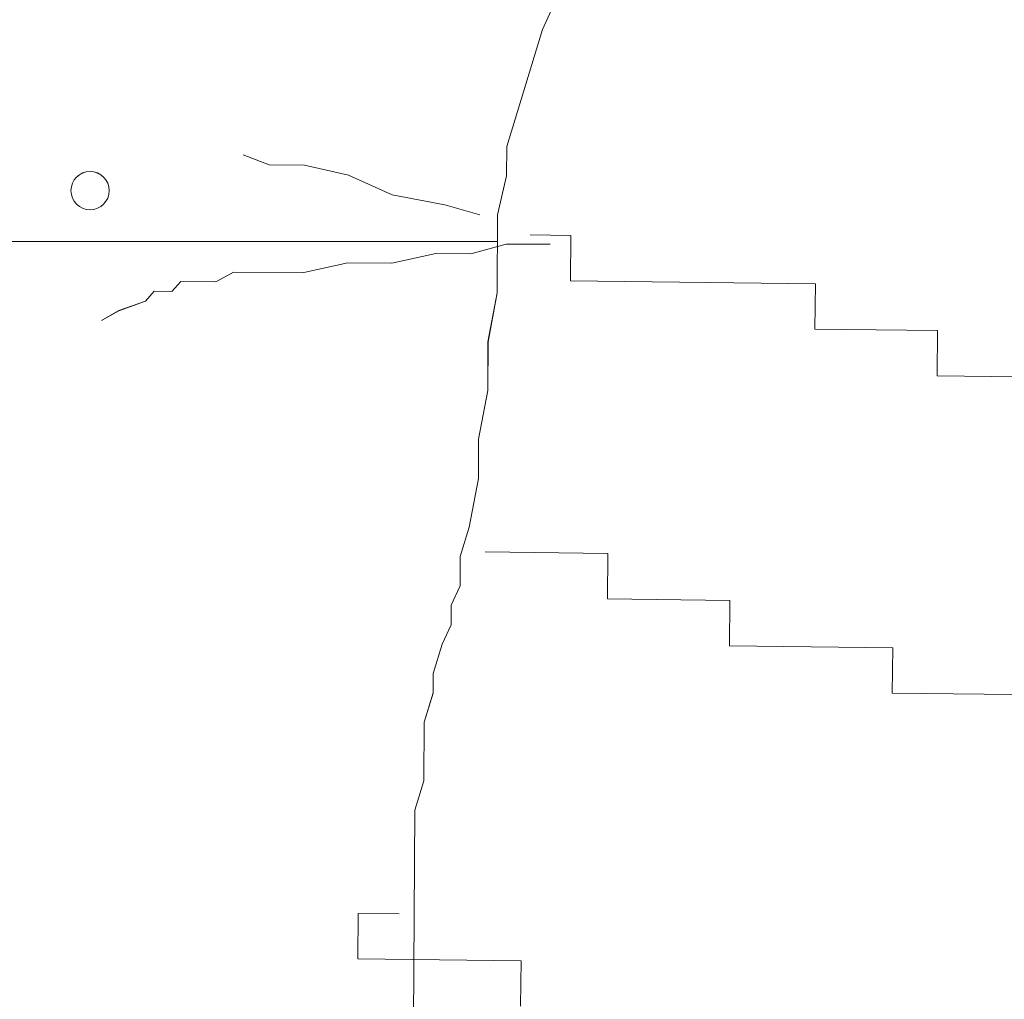
# Model space of a CAD drawing. Units: inches. Extents: x -466983 to 1020, y 324 to 318697.
# Tile 59 of 97: x 631.804 to 634.801, y 942.694 to 945.675. Entities that reach past the tile are written whole.
import ezdxf

# ---------------------------------------------------------------- set-up
doc = ezdxf.new("R2010")
doc.units = ezdxf.units.IN
doc.header["$MEASUREMENT"] = 0
doc.layers.add('A-FLOR-PATT', color=252, linetype='Continuous', lineweight=13)
doc.layers.add('A-FURN', color=8, linetype='Continuous', lineweight=18)

# ---------------------------------------------------------------- blocks, each defined once
blk = doc.blocks.new('L Shaped Sofa')
at = {"ltscale": 2}
for p, q in [((2438.4141, 742.6892), (2438.4273, 744.8578)), ((2437.8266, 743.7781), (2437.8235, 743.5262)), ((2437.8235, 743.5262), (2438.7308, 743.5151)), ((2438.7308, 743.5151), (2438.7278, 743.2632)), ((2438.7278, 743.2632), (2438.5009, 743.2659)), ((2438.3643, 742.5267), (2438.4141, 742.6892)), ((2438.3623, 742.2015), (2438.3643, 742.5267)), ((2438.3125, 742.039), (2438.3623, 742.2015)), ((2435.083, 742.048), (2435.7635, 742.0396)), ((2435.7635, 742.0396), (2435.7604, 741.7877)), ((2438.3118, 741.9306), (2438.3125, 742.039)), ((2438.262, 741.7682), (2438.3118, 741.9306)), ((2435.7604, 741.7877), (2436.6678, 741.7766)), ((2436.6678, 741.7766), (2436.6647, 741.5247)), ((2438.2126, 741.66), (2438.262, 741.7682)), ((2438.2119, 741.5515), (2438.2126, 741.66)), ((2438.1624, 741.4433), (2438.2119, 741.5515)), ((2436.6647, 741.5247), (2437.3452, 741.5164)), ((2437.3452, 741.5164), (2437.3421, 741.2645)), ((2438.1615, 741.2807), (2438.1624, 741.4433)), ((2438.1117, 741.1183), (2438.1615, 741.2807)), ((2437.3421, 741.2645), (2438.0226, 741.2562)), ((2438.0612, 740.8474), (2438.1117, 741.1183)), ((2438.0599, 740.6306), (2438.0612, 740.8474)), ((2438.0094, 740.3597), (2438.0599, 740.6306)), ((2438.0078, 740.0886), (2438.0094, 740.3597)), ((2435.0614, 740.2846), (2435.5151, 740.279)), ((2435.5151, 740.279), (2435.512, 740.0271)), ((2437.9573, 739.8178), (2438.0078, 740.0886)), ((2435.512, 740.0271), (2436.1926, 740.0188)), ((2436.1926, 740.0188), (2436.1895, 739.7669)), ((2440.0562, 739.9164), (2440.1541, 739.9701)), ((2439.9094, 739.8628), (2440.0562, 739.9164)), ((2439.8603, 739.8089), (2439.9094, 739.8628)), ((2437.9547, 739.3841), (2437.9573, 739.8178)), ((2439.7136, 739.7553), (2439.7627, 739.8093)), ((2439.7627, 739.8093), (2439.8603, 739.8089)), ((2436.1895, 739.7669), (2437.5505, 739.7503)), ((2437.5505, 739.7503), (2437.5474, 739.4984)), ((2439.4205, 739.7025), (2439.5184, 739.7562)), ((2439.5184, 739.7562), (2439.7136, 739.7553)), ((2438.7858, 739.6512), (2439.0301, 739.7043)), ((2439.0301, 739.7043), (2439.4205, 739.7025)), ((2438.2975, 739.5993), (2438.5419, 739.6524)), ((2438.5419, 739.6524), (2438.7858, 739.6512)), ((2437.9069, 739.5469), (2438.1024, 739.6002)), ((2438.1024, 739.6002), (2438.2975, 739.5993)), ((2437.6629, 739.5481), (2437.9069, 739.5469)), ((2458.9601, 739.5321), (2437.9556, 739.5321)), ((2437.5474, 739.4984), (2437.7743, 739.4956)), ((2437.9045, 739.1674), (2437.9547, 739.3841)), ((2438.0522, 739.3836), (2438.2471, 739.3285)), ((2438.2471, 739.3285), (2438.5395, 739.2729)), ((2438.5395, 739.2729), (2438.7828, 739.1633)), ((2437.9035, 739.0048), (2437.9045, 739.1674)), ((2438.7828, 739.1633), (2439.0265, 739.1079)), ((2439.0265, 739.1079), (2439.2217, 739.107)), ((2439.2217, 739.107), (2439.3677, 739.0521)), ((2437.7044, 738.3551), (2437.9035, 739.0048)), ((2437.6549, 738.2469), (2437.7044, 738.3551))]:
    blk.add_line(p, q, dxfattribs=at)
for start, end in [(90, 270), (270, 90)]:
    blk.add_arc((2440.2165, 739.2499), 0.1062, start, end, dxfattribs=at)

msp = doc.modelspace()

# ---------------------------------------------------------------- hatches: boundary and pattern name
at = {"layer": 'A-FLOR-PATT', "transparency": 33554572}
h = msp.add_hatch(dxfattribs=at)
h.set_pattern_fill('ANSI37', color=256, scale=30)
h.set_pattern_definition([(45, (-1212.4137, -290.035), (-2.6516504, 2.6516504), []), (135, (-1212.4137, -290.035), (-2.6516504, -2.6516504), [])])
h.paths.add_polyline_path([(901.8057, 1075.9377), (900.6144, 1075.9377), (900.6144, 1065.3856), (899.391, 1065.3856), (898.0911, 1065.3856), (892.8356, 1058.7098, -0.258377), (892.1875, 1058.3509), (879.9848, 1058.3509, -0.20177), (879.4382, 1058.5808), (874.0812, 1065.3856), (872.7813, 1065.3856), (871.5579, 1065.3856), (871.5579, 1075.9377), (813.8057, 1075.9377), (813.8057, 1044.7922), (832.3947, 1044.7922, -0.394795), (848.6602, 1028.5356), (848.6602, 1009.9377), (901.8057, 1009.9377), (901.8057, 1015.9377), (901.3057, 1015.9377), (871.3057, 1015.9377), (871.3057, 1017.2502), (871.3344, 1017.2502, -0.401453), (901.3057, 1045.9377), (901.8057, 1045.9377)])
edge = h.paths.add_edge_path(flags=16)
edge.add_line((847.7731, 1068.9486), (847.7731, 1073.7088))
edge.add_arc((849.2269, 1073.7088), 1.4538, 90, 180, ccw=False)
edge.add_line((849.2269, 1075.1627), (864.4921, 1075.1627))
edge.add_arc((864.4921, 1073.7088), 1.4538, 0, 90, ccw=False)
edge.add_line((865.9459, 1073.7088), (865.9459, 1069.0035))
edge.add_arc((832.6447, 1068.9761), 33.3012, -20.61234, 0.04725, ccw=False)
edge.add_ellipse((856.8595, 1058.48), major_axis=(0, 10.2131), ratio=0.6859192, start_angle=100.00884, end_angle=259.99116, ccw=False)
edge.add_arc((881.0742, 1068.9761), 33.3012, 180.04725, 200.61234, ccw=False)
h.paths.add_polyline_path([(853.1456, 1066.4815), (853.1456, 1066.4534), (853.1463, 1066.4534, 0.433107), (852.9166, 1066.6849), (852.9166, 1066.4534), (853.1456, 1066.4534), (853.1456, 1066.4815), (853.088, 1066.6122, 0.697939), (852.6995, 1066.4534), (852.7003, 1066.4534), (852.7003, 1066.4815), (852.9166, 1067.0012), (852.9166, 1066.6849, -0.396254)], flags=0)
h.paths.add_polyline_path([(861.0187, 1066.4815), (861.0187, 1066.4534), (861.0194, 1066.4534, 0.416404), (860.8024, 1066.6849), (860.8024, 1066.4534), (861.0187, 1066.4534), (861.0187, 1066.4815), (860.9672, 1066.6053, 0.713344), (860.5726, 1066.4534), (860.5734, 1066.4534), (860.5734, 1066.4815), (860.8024, 1067.0012), (860.8024, 1066.6849, -0.379973)], flags=0)
edge = h.paths.add_edge_path(flags=0)
edge.add_spline(control_points=[(861.1298, 1065.7855), (861.4661, 1065.2478), (861.6134, 1065.0161), (861.9833, 1064.3736), (862.1924, 1063.9443), (862.5614, 1063.0391), (862.7212, 1062.5633), (862.9865, 1061.5781), (863.092, 1061.0689), (863.2452, 1060.031), (863.293, 1059.5025), (863.3295, 1058.4409), (863.3181, 1057.9078), (863.2366, 1056.8518), (863.1664, 1056.3289), (862.9695, 1055.308), (862.8427, 1054.8099), (862.5365, 1053.8522), (862.3571, 1053.3927), (861.9514, 1052.5249), (861.7251, 1052.1166), (861.233, 1051.3622), (860.9672, 1051.0162), (860.4048, 1050.3949), (860.1082, 1050.1197), (859.4937, 1049.6461), (859.1758, 1049.4476), (858.5276, 1049.1299), (858.1973, 1049.0107), (857.5315, 1048.8518), (857.1959, 1048.8121), (856.5249, 1048.812), (856.1894, 1048.8515), (855.5236, 1049.0101), (855.1933, 1049.1291), (854.545, 1049.4465), (854.2271, 1049.6449), (853.6124, 1050.1183), (853.3158, 1050.3933), (852.7533, 1051.0143), (852.4874, 1051.3602), (851.9952, 1052.1144), (851.7688, 1052.5225), (851.3629, 1053.3902), (851.1834, 1053.8496), (850.877, 1054.8071), (850.7501, 1055.3051), (850.553, 1056.326), (850.4827, 1056.8488), (850.401, 1057.9048), (850.3895, 1058.4379), (850.4257, 1059.4995), (850.4734, 1060.0281), (850.6265, 1061.066), (850.7318, 1061.5753), (850.9969, 1062.5605), (851.1567, 1063.0365), (851.5254, 1063.9418), (851.7345, 1064.3712), (852.1056, 1065.0164), (852.2544, 1065.2503), (852.6082, 1065.7335)], knot_values=[3.915332, 3.915332, 3.915332, 3.915332, 4.013468, 4.013468, 4.175532, 4.175532, 4.337596, 4.337596, 4.49966, 4.49966, 4.661724, 4.661724, 4.823788, 4.823788, 4.985852, 4.985852, 5.147916, 5.147916, 5.30998, 5.30998, 5.472044, 5.472044, 5.634109, 5.634109, 5.796173, 5.796173, 5.958237, 5.958237, 6.120301, 6.120301, 6.282365, 6.282365, 6.444429, 6.444429, 6.606493, 6.606493, 6.768557, 6.768557, 6.930621, 6.930621, 7.092685, 7.092685, 7.254749, 7.254749, 7.416813, 7.416813, 7.578878, 7.578878, 7.740942, 7.740942, 7.903006, 7.903006, 8.06507, 8.06507, 8.227134, 8.227134, 8.389198, 8.389198, 8.551262, 8.551262, 8.65037, 8.65037, 8.65037, 8.65037], degree=3, periodic=0)
edge.add_line((852.6421, 1065.7855), (861.1298, 1065.7855))
edge = h.paths.add_edge_path(flags=0)
edge.add_ellipse((856.8496, 1057.7432), major_axis=(0, 7.7921), ratio=0.687861, start_angle=0, end_angle=360)
h.paths.add_polyline_path([(848.8634, 1069.3891), (848.8634, 1073.9605, -0.414214), (849.9538, 1075.0508), (863.7652, 1075.0508, -0.414214), (864.8555, 1073.9605), (864.8555, 1069.3891, -0.388936), (864.5237, 1069.027, -0.043561), (849.1953, 1069.027, -0.388936)], flags=0)
h.paths.add_polyline_path([(853.1006, 1068.1122, -1), (852.6775, 1068.1122, -1)], flags=0)
edge = h.paths.add_edge_path(flags=0)
edge.add_ellipse((856.8595, 1057.3378), major_axis=(0, 2.207), ratio=0.657164, start_angle=0, end_angle=360)
h.paths.add_polyline_path([(861.0415, 1068.1122, -1), (860.6184, 1068.1122, -1)], flags=0)
edge = h.paths.add_edge_path()
edge.add_line((573.9537, 1057.3412), (573.9537, 1075.9377))
edge.add_line((573.9537, 1075.9377), (558.7308, 1075.9377))
edge.add_line((558.7308, 1075.9377), (558.7308, 1065.3856))
edge.add_line((558.7308, 1065.3856), (557.5074, 1065.3856))
edge.add_line((557.5074, 1065.3856), (556.2075, 1065.3856))
edge.add_line((556.2075, 1065.3856), (550.952, 1058.7098))
edge.add_arc((550.3039, 1059.1155), 0.7646, 270, 327.9483, ccw=False)
edge.add_line((550.3039, 1058.3509), (538.1012, 1058.3509))
edge.add_arc((538.1012, 1059.1155), 0.7646, 224.3704, 270, ccw=False)
edge.add_line((537.5546, 1058.5808), (532.1976, 1065.3856))
edge.add_line((532.1976, 1065.3856), (530.8977, 1065.3856))
edge.add_line((530.8977, 1065.3856), (529.6743, 1065.3856))
edge.add_line((529.6743, 1065.3856), (529.6743, 1075.9377))
edge.add_line((529.6743, 1075.9377), (520.8057, 1075.9377))
edge.add_line((520.8057, 1075.9377), (520.8057, 1045.9377))
edge.add_line((520.8057, 1045.9377), (521.3057, 1045.9377))
edge.add_arc((521.3057, 1015.9377), 30, 2.50749, 90, ccw=False)
edge.add_line((551.277, 1017.2502), (551.3057, 1017.2502))
edge.add_line((551.3057, 1017.2502), (551.3057, 1015.9377))
edge.add_line((551.3057, 1015.9377), (520.8057, 1015.9377))
edge.add_line((520.8057, 1015.9377), (520.8057, 1009.9377))
edge.add_line((520.8057, 1009.9377), (559.1913, 1010.4022))
edge.add_arc((559.1913, 1011.856), 1.4538, 180, 270, ccw=False)
edge.add_line((557.7375, 1011.856), (557.7375, 1016.5613))
edge.add_arc((591.0386, 1016.5888), 33.3012, 159.38766, 180.04725, ccw=False)
edge.add_ellipse((566.8239, 1027.0848), major_axis=(0, 10.2131), ratio=0.6859192, start_angle=280.00884, end_angle=439.99116, ccw=False)
edge.add_arc((542.6091, 1016.5888), 33.3012, 0.04725, 20.61234, ccw=False)
edge.add_line((575.9103, 1016.6162), (575.9103, 1011.856))
edge.add_arc((574.4565, 1011.856), 1.4538, -90, 0, ccw=False)
edge.add_line((574.4565, 1010.4022), (608.8057, 1009.9377))
edge.add_line((608.8057, 1009.9377), (608.8057, 1041.0857))
edge.add_line((608.8057, 1041.0857), (590.2179, 1041.0857))
edge.add_arc((590.775, 1057.9074), 16.8309, 181.92775, 268.10321, ccw=False)
edge = h.paths.add_edge_path()
edge.add_ellipse((494.2443, 583.6204), major_axis=(0, 10.2131), ratio=0.6859192, start_angle=280.00884, end_angle=439.99116, ccw=False)
edge.add_arc((470.0296, 573.1243), 33.3012, 0.04725, 20.61234, ccw=False)
edge.add_line((503.3307, 573.1518), (503.3307, 568.3916))
edge.add_arc((501.8769, 568.3916), 1.4538, -90, 0, ccw=False)
edge.add_line((501.8769, 566.9377), (539.8057, 566.9377))
edge.add_line((539.8057, 566.9377), (539.8057, 572.9377))
edge.add_line((539.8057, 572.9377), (539.3057, 572.9377))
edge.add_line((539.3057, 572.9377), (509.3057, 572.9377))
edge.add_line((509.3057, 572.9377), (509.3057, 574.2502))
edge.add_line((509.3057, 574.2502), (509.3344, 574.2502))
edge.add_arc((539.3057, 572.9377), 30, 90, 177.49251, ccw=False)
edge.add_line((539.3057, 602.9377), (539.8057, 602.9377))
edge.add_line((539.8057, 602.9377), (539.8057, 626.9377))
edge.add_line((539.8057, 626.9377), (531.7718, 626.9377))
edge.add_line((531.7718, 626.9377), (531.7718, 616.3856))
edge.add_line((531.7718, 616.3856), (530.5484, 616.3856))
edge.add_line((530.5484, 616.3856), (529.2485, 616.3856))
edge.add_line((529.2485, 616.3856), (523.7105, 609.3509))
edge.add_line((523.7105, 609.3509), (510.7766, 609.3509))
edge.add_line((510.7766, 609.3509), (505.2386, 616.3856))
edge.add_line((505.2386, 616.3856), (503.9387, 616.3856))
edge.add_line((503.9387, 616.3856), (502.7153, 616.3856))
edge.add_line((502.7153, 616.3856), (502.7153, 626.9377))
edge.add_line((502.7153, 626.9377), (481.6983, 626.9377))
edge.add_line((481.6983, 626.9377), (481.6983, 610.995))
edge.add_arc((467.2703, 611.4728), 14.4359, 271.92775, 358.10321, ccw=False)
edge.add_line((467.7559, 597.0451), (451.8057, 597.0451))
edge.add_line((451.8057, 597.0451), (451.8057, 584.4035))
edge.add_line((451.8057, 584.4035), (451.8057, 566.9377))
edge.add_line((451.8057, 566.9377), (486.6117, 566.9377))
edge.add_arc((486.6117, 568.3916), 1.4538, 180, 270, ccw=False)
edge.add_line((485.1579, 568.3916), (485.1579, 573.0969))
edge.add_arc((518.4591, 573.1243), 33.3012, 159.38766, 180.04725, ccw=False)
h.paths.add_polyline_path([(836.2609, 1020.7328), (879.8898, 1020.7328), (879.8898, 1039.3902), (836.2609, 1039.3902)], flags=25)
h.paths.add_polyline_path([(549.9851, 1036.7492), (593.614, 1036.7492), (593.614, 1055.4065), (549.9851, 1055.4065)], flags=24)
h.paths.add_polyline_path([(475.123, 595.5959), (518.752, 595.5959), (518.752, 614.2532), (475.123, 614.2532)], flags=24)
h = msp.add_hatch(dxfattribs=at)
h.set_pattern_fill('ANSI37', color=256, scale=20)
h.set_pattern_definition([(45, (-1212.4137, -290.035), (-1.767767, 1.767767), []), (135, (-1212.4137, -290.035), (-1.767767, -1.767767), [])])
h.paths.add_polyline_path([(809.8057, 870.9377), (809.8057, 888.1519), (806.9985, 888.1519), (802.6624, 888.1519), (789.3832, 888.1519), (786.2846, 888.1519, -0.414214), (785.4991, 888.9374), (785.4991, 900.1959), (785.4991, 908.4696, -0.414214), (786.8082, 909.7787, -0.414214), (785.4991, 911.0878), (785.4991, 929.1015, -0.414214), (786.8082, 930.4106, -0.414214), (785.4991, 931.7197), (785.4991, 931.9039, -0.414214), (784.19, 930.5948), (766.7223, 930.5948, -0.412359), (765.4132, 931.8956, -0.413741), (764.1145, 930.5782), (744.5781, 930.422, -0.416556), (743.7864, 931.2075), (743.7864, 933.5153), (742.2154, 933.5153), (742.2154, 952.024, -0.001344), (743.7864, 952.1998), (743.7864, 953.9377), (678.5915, 953.9377), (678.5915, 951.1305), (678.5915, 946.7945), (678.5915, 933.5153), (678.5915, 930.4166, -0.414214), (677.806, 929.6312), (666.5475, 929.6312), (658.2738, 929.6312, -0.414214), (656.9647, 930.9403, -0.414214), (655.6556, 929.6312), (637.6419, 929.6312, -0.414214), (636.3328, 930.9403, -0.414214), (635.0237, 929.6312), (634.8395, 929.6312, -0.414214), (636.1486, 928.322), (636.1486, 910.8544, -0.412359), (634.8478, 909.5452, -0.413741), (636.1653, 908.2466), (636.3214, 888.7102, -0.416556), (635.5359, 887.9184), (633.2281, 887.9184), (633.2281, 886.3475), (614.7194, 886.3475, -0.001344), (614.5436, 887.9184), (612.8057, 887.9184), (612.8057, 834.9377), (612.8057, 752.9377), (612.8057, 748.9377), (612.8057, 697.9377), (654.8057, 697.9377), (654.8057, 701.9377), (715.8057, 701.9377), (715.8057, 737.4353), (774.2918, 737.4353), (774.2918, 795.9377), (809.8057, 795.9377)])
h.paths.add_polyline_path([(679.2761, 849.5757, 0.102523), (682.1475, 849.2608, -0.080461), (694.5428, 849.7725, -0.283899), (694.4822, 849.0082, 0.136605), (694.4068, 848.8103, -0.030441), (694.5428, 846.8929), (694.5428, 842.6198), (694.5428, 838.3466, -0.028219), (694.4246, 836.5684), (694.425, 836.5684, 0.196187), (694.4456, 836.2708, -0.302897), (694.5428, 835.467, -0.080461), (682.1475, 835.9787, 0.102523), (679.2761, 835.6638, -0.58611), (678.6457, 836.0169), (678.6457, 849.2227, -0.58611)], flags=16)
h.paths.add_polyline_path([(679.5173, 848.6515, 0.699597), (679.476, 848.6342, 1.20716), (679.1935, 848.7422, 0.010621)], flags=0)
h.paths.add_polyline_path([(679.4923, 836.5608, -0.013798), (679.9178, 836.6594, -0.071703), (682.8533, 837.1434, -0.165743), (682.1665, 839.1006), (682.1665, 842.6094), (682.1665, 846.0603, -0.240616), (683.4733, 848.6767, -0.068263), (693.9295, 849.0082), (693.7875, 848.7083), (693.7875, 849.0228, 0.067332), (683.4733, 848.6767, 0.240616), (682.1665, 846.0603), (682.1665, 842.6094), (682.1665, 839.1006, 0.23459), (683.461, 836.5513, 0.068093), (693.7875, 836.1955), (693.7875, 836.5104), (693.9296, 836.2102, -0.077215), (682.2421, 836.7815, 0.086627), (679.5283, 836.5701, -0.628402), (679.5029, 836.5735), (679.5029, 836.6071, 0.910458)], flags=0)
h.paths.add_polyline_path([(679.476, 848.6364), (679.2069, 848.647), (679.2069, 836.5718, 0.913566), (679.3645, 836.5861), (679.476, 836.5824)], flags=0)
h.paths.add_polyline_path([(679.2761, 829.8604, 0.102523), (682.1475, 829.5455, -0.080461), (694.5428, 830.0572, -0.283899), (694.4822, 829.2929, 0.136605), (694.4068, 829.095, -0.030441), (694.5428, 827.1776), (694.5428, 822.9045), (694.5428, 818.6314, -0.028219), (694.4246, 816.8531), (694.425, 816.8532, 0.196187), (694.4456, 816.5555, -0.302897), (694.5428, 815.7517, -0.080461), (682.1475, 816.2635, 0.102523), (679.2761, 815.9485, -0.58611), (678.6457, 816.3016), (678.6457, 829.5074, -0.58611)], flags=16)
h.paths.add_polyline_path([(679.5173, 828.9362, 0.699597), (679.476, 828.9189, 1.20716), (679.1935, 829.0269, 0.010621)], flags=0)
h.paths.add_polyline_path([(679.4923, 816.8456, -0.013798), (679.9178, 816.9441, -0.071703), (682.8533, 817.4281, -0.165743), (682.1665, 819.3853), (682.1665, 822.8941), (682.1665, 826.345, -0.240616), (683.4733, 828.9614, -0.068263), (693.9295, 829.2929), (693.7875, 828.9931), (693.7875, 829.3076, 0.067332), (683.4733, 828.9614, 0.240616), (682.1665, 826.345), (682.1665, 822.8941), (682.1665, 819.3853, 0.23459), (683.461, 816.836, 0.068093), (693.7875, 816.4802), (693.7875, 816.7952), (693.9296, 816.4949, -0.077215), (682.2421, 817.0662, 0.086627), (679.5283, 816.8549, -0.628402), (679.5029, 816.8582), (679.5029, 816.8918, 0.910458)], flags=0)
h.paths.add_polyline_path([(679.476, 828.9211), (679.2069, 828.9317), (679.2069, 816.8565, 0.913566), (679.3645, 816.8708), (679.476, 816.8671)], flags=0)
h.paths.add_polyline_path([(679.2761, 810.1451, 0.102523), (682.1475, 809.8302, -0.080461), (694.5428, 810.342, -0.3023), (694.4466, 809.5394, 0.10023), (694.4058, 809.3878, -0.03057), (694.5428, 807.4623), (694.5428, 803.1892), (694.5428, 798.9161, -0.03057), (694.4058, 796.9906, 0.10023), (694.4466, 796.839, -0.3023), (694.5428, 796.0365, -0.080461), (682.1475, 796.5482, 0.102523), (679.2761, 796.2333, -0.58611), (678.6457, 796.5863), (678.6457, 809.7921, -0.58611)], flags=16)
h.paths.add_polyline_path([(679.5173, 809.2417, 0.699597), (679.476, 809.2244, 1.20716), (679.1935, 809.3324, 0.010621)], flags=0)
h.paths.add_polyline_path([(679.4923, 797.151, -0.013798), (679.9178, 797.2496, -0.071703), (682.8533, 797.7336, -0.165743), (682.1665, 799.6908), (682.1665, 803.1996), (682.1665, 806.6505, -0.239349), (683.461, 809.2577, -0.072465), (694.4468, 809.5405, 0.197932), (694.425, 809.2405), (693.7875, 809.2985), (693.7875, 809.6135, 0.068093), (683.461, 809.2577, 0.239349), (682.1665, 806.6505), (682.1665, 803.1996), (682.1665, 799.6908, 0.235854), (683.4733, 797.1323, 0.067332), (693.7875, 796.7861), (693.7875, 797.1006), (694.425, 797.1586, 0.197932), (694.4468, 796.8586, -0.080419), (682.1557, 797.3795, 0.083867), (679.5283, 797.1603, -0.628402), (679.5029, 797.1637), (679.5029, 797.1973, 0.910458)], flags=0)
h.paths.add_polyline_path([(679.2069, 809.2372), (679.2069, 797.162, 0.913566), (679.3645, 797.1763), (679.476, 797.1726), (679.476, 809.2266)], flags=0)
h.paths.add_polyline_path([(695.3643, 853.2989), (728.2231, 853.2989), (728.2231, 771.1519), (695.3643, 771.1519)], flags=16)
h.paths.add_polyline_path([(696.0215, 852.6417), (727.5659, 852.6417), (727.5659, 771.809), (696.0215, 771.809)], flags=0)
h.paths.add_polyline_path([(679.2761, 788.7869, 0.102523), (682.1475, 788.472, -0.080461), (694.5428, 788.9837, -0.3023), (694.4466, 788.1812, 0.10023), (694.4058, 788.0296, -0.03057), (694.5428, 786.1041), (694.5428, 781.831), (694.5428, 777.5578, -0.03057), (694.4058, 775.6323, 0.10023), (694.4466, 775.4808, -0.3023), (694.5428, 774.6782, -0.080461), (682.1475, 775.19, 0.102523), (679.2761, 774.875, -0.58611), (678.6457, 775.2281), (678.6457, 788.4339, -0.58611)], flags=16)
h.paths.add_polyline_path([(679.5173, 787.8834, 0.699597), (679.476, 787.8662, 1.20716), (679.1935, 787.9742, 0.010621)], flags=0)
h.paths.add_polyline_path([(679.4923, 775.7928, -0.013798), (679.9178, 775.8914, -0.071703), (682.8533, 776.3753, -0.165743), (682.1665, 778.3325), (682.1665, 781.8414), (682.1665, 785.2922, -0.239349), (683.461, 787.8995, -0.072465), (694.4468, 788.1823, 0.197932), (694.425, 787.8823), (693.7875, 787.9403), (693.7875, 788.2553, 0.068093), (683.461, 787.8995, 0.239349), (682.1665, 785.2922), (682.1665, 781.8414), (682.1665, 778.3325, 0.235854), (683.4733, 775.7741, 0.067332), (693.7875, 775.4279), (693.7875, 775.7424), (694.425, 775.8004, 0.197932), (694.4468, 775.5004, -0.080419), (682.1557, 776.0212, 0.083867), (679.5283, 775.8021, -0.628402), (679.5029, 775.8054), (679.5029, 775.8391, 0.910458)], flags=0)
h.paths.add_polyline_path([(679.2069, 787.8789), (679.2069, 775.8038, 0.913566), (679.3645, 775.818), (679.476, 775.8144), (679.476, 787.8684)], flags=0)
h.paths.add_polyline_path([(704.641, 854.1204, -0.080461), (705.1527, 866.5157, 0.102523), (704.8378, 869.3871, -0.58611), (705.1908, 870.0174), (718.3966, 870.0174, -0.58611), (718.7496, 869.3871, 0.102523), (718.4347, 866.5157, -0.080461), (718.9465, 854.1204, -0.3023), (718.1439, 854.2166, 0.10023), (717.9924, 854.2574, -0.03057), (716.0668, 854.1204), (711.7937, 854.1204), (707.5206, 854.1204, -0.03057), (705.5951, 854.2574, 0.10023), (705.4435, 854.2166, -0.3023)], flags=16)
h.paths.add_polyline_path([(717.8462, 869.1459, 0.699597), (717.8289, 869.1872, 1.20716), (717.9369, 869.4697, 0.010621)], flags=0)
h.paths.add_polyline_path([(705.4631, 854.2164, -0.080419), (705.984, 866.5074, 0.083867), (705.7648, 869.1349, -0.628402), (705.7682, 869.1603), (705.8018, 869.1603, 0.910458), (705.7555, 869.1709, -0.013798), (705.8541, 868.7454, -0.071703), (706.3381, 865.8099, -0.165743), (708.2953, 866.4967), (711.8041, 866.4967), (715.255, 866.4967, -0.239349), (717.8622, 865.2022, -0.072465), (718.145, 854.2164, 0.197932), (717.845, 854.2382), (717.903, 854.8757), (718.218, 854.8757, 0.068093), (717.8622, 865.2022, 0.239349), (715.255, 866.4967), (711.8041, 866.4967), (708.2953, 866.4967, 0.235854), (705.7368, 865.1898, 0.067332), (705.3906, 854.8757), (705.7051, 854.8757), (705.7631, 854.2382, 0.197932)], flags=16)
h.paths.add_polyline_path([(705.7665, 869.4563, 0.913566), (705.7808, 869.2987), (705.7771, 869.1872), (717.8311, 869.1872), (717.8417, 869.4563)], flags=0)
h.paths.add_polyline_path([(729.0446, 842.6198), (729.0446, 846.8929, -0.03057), (729.1817, 848.8184, 0.10023), (729.1408, 848.9699, -0.3023), (729.0446, 849.7725, -0.080461), (741.4399, 849.2608, 0.102523), (744.3113, 849.5757, -0.58611), (744.9417, 849.2227), (744.9417, 836.0169, -0.58611), (744.3113, 835.6638, 0.102523), (741.4399, 835.9787, -0.080461), (729.0446, 835.467, -0.3023), (729.1408, 836.2696, 0.10023), (729.1817, 836.4211, -0.03057), (729.0446, 838.3466)], flags=16)
h.paths.add_polyline_path([(744.1115, 836.5846, 1.20716), (744.3939, 836.4766, 0.010621), (744.0701, 836.5673, 0.699597)], flags=0)
h.paths.add_polyline_path([(729.1407, 836.2684, 0.197932), (729.1624, 836.5684), (729.7999, 836.5104), (729.7999, 836.1955, 0.068093), (740.1264, 836.5513, 0.239349), (741.4209, 839.1585), (741.4209, 842.6094), (741.4209, 846.1182, 0.235854), (740.1141, 848.6767, 0.067332), (729.7999, 849.0228), (729.7999, 848.7083), (729.1624, 848.6503, 0.197932), (729.1407, 848.9504, -0.080419), (741.4317, 848.4295, 0.083867), (744.0591, 848.6486, -0.628402), (744.0845, 848.6453), (744.0845, 848.6117, 0.910458), (744.0951, 848.6579, -0.013798), (743.6696, 848.5594, -0.071703), (740.7341, 848.0754, -0.165743), (741.4209, 846.1182), (741.4209, 842.6094), (741.4209, 839.1585, -0.239349), (740.1264, 836.5513, -0.072465)], flags=0)
h.paths.add_polyline_path([(729.0446, 830.0572, -0.080461), (741.4399, 829.5455, 0.102523), (744.3113, 829.8604, -0.58611), (744.9417, 829.5074), (744.9417, 816.3016, -0.58611), (744.3113, 815.9485, 0.102523), (741.4399, 816.2635, -0.080461), (729.0446, 815.7517, -0.3023), (729.1408, 816.5543, 0.10023), (729.1817, 816.7058, -0.03057), (729.0446, 818.6314), (729.0446, 822.9045), (729.0446, 827.1776, -0.03057), (729.1817, 829.1031, 0.10023), (729.1408, 829.2547, -0.3023)], flags=16)
h.paths.add_polyline_path([(744.1115, 816.8693, 1.20716), (744.3939, 816.7613, 0.010621), (744.0701, 816.852, 0.699597)], flags=0)
h.paths.add_polyline_path([(729.1407, 829.2351, -0.080419), (741.4317, 828.7142, 0.083867), (744.0591, 828.9334, -0.628402), (744.0845, 828.93), (744.0845, 828.8964, 0.910458), (744.0951, 828.9427, -0.013798), (743.6696, 828.8441, -0.071703), (740.7341, 828.3601, -0.165743), (741.4209, 826.4029), (741.4209, 822.8941), (741.4209, 819.4432, -0.239349), (740.1264, 816.836, -0.072465), (729.1407, 816.5531, 0.197932), (729.1624, 816.8532), (729.7999, 816.7952), (729.7999, 816.4802, 0.068093), (740.1264, 816.836, 0.239349), (741.4209, 819.4432), (741.4209, 822.8941), (741.4209, 826.4029, 0.235854), (740.1141, 828.9614, 0.067332), (729.7999, 829.3076), (729.7999, 828.9931), (729.1624, 828.9351, 0.197932)], flags=16)
h.paths.add_polyline_path([(729.0446, 810.342, -0.080461), (741.4399, 809.8302, 0.102523), (744.3113, 810.1451, -0.58611), (744.9417, 809.7921), (744.9417, 796.5863, -0.58611), (744.3113, 796.2333, 0.102523), (741.4399, 796.5482, -0.080461), (729.0446, 796.0365, -0.283899), (729.1052, 796.8007, 0.136605), (729.1806, 796.9987, -0.030441), (729.0446, 798.9161), (729.0446, 803.1892), (729.0446, 807.4623, -0.028219), (729.1628, 809.2406), (729.1624, 809.2405, 0.196187), (729.1418, 809.5382, -0.302897)], flags=16)
h.paths.add_polyline_path([(744.1115, 797.1748, 1.20716), (744.3939, 797.0668, 0.010621), (744.0701, 797.1575, 0.699597)], flags=0)
h.paths.add_polyline_path([(741.3453, 809.0275, 0.086627), (744.0591, 809.2388, -0.628402), (744.0845, 809.2355), (744.0845, 809.2019, 0.910458), (744.0951, 809.2481, -0.013798), (743.6696, 809.1496, -0.071703), (740.7341, 808.6656, -0.165743), (741.4209, 806.7084), (741.4209, 803.1996), (741.4209, 799.7487, -0.240616), (740.1141, 797.1323, -0.068263), (729.658, 796.8008), (729.7999, 797.1006), (729.7999, 796.7861, 0.067332), (740.1141, 797.1323, 0.240616), (741.4209, 799.7487), (741.4209, 803.1996), (741.4209, 806.7084, 0.23459), (740.1264, 809.2577, 0.068093), (729.7999, 809.6135), (729.7999, 809.2985), (729.6578, 809.5988, -0.077215)], flags=0)
h.paths.add_polyline_path([(704.641, 770.3304, -0.283899), (705.4053, 770.2697, 0.136605), (705.6032, 770.1944, -0.030441), (707.5206, 770.3304), (711.7937, 770.3304), (716.0668, 770.3304, -0.028219), (717.8451, 770.2122), (717.845, 770.2126, 0.196187), (718.1427, 770.2331, -0.302897), (718.9465, 770.3304, -0.080461), (718.4347, 757.9351, 0.102523), (718.7496, 755.0637, -0.58611), (718.3966, 754.4333), (705.1908, 754.4333, -0.58611), (704.8378, 755.0637, 0.102523), (705.1527, 757.9351, -0.080461)], flags=16)
h.paths.add_polyline_path([(705.762, 755.3048, 0.699597), (705.7793, 755.2635, 1.20716), (705.6713, 754.9811, 0.010621)], flags=0)
h.paths.add_polyline_path([(705.4053, 769.717), (705.7051, 769.5751), (705.3906, 769.5751, 0.067332), (705.7368, 759.2609, 0.240616), (708.3532, 757.954), (711.8041, 757.954), (715.3129, 757.954, 0.23459), (717.8622, 759.2485, 0.068093), (718.218, 769.5751), (717.903, 769.5751), (718.2033, 769.7172, -0.077215), (717.632, 758.0297, 0.086627), (717.8433, 755.3159, -0.628402), (717.84, 755.2904), (717.8064, 755.2904, 0.910458), (717.8526, 755.2799, -0.013798), (717.7541, 755.7053, -0.071703), (717.2701, 758.6409, -0.165743), (715.3129, 757.954), (711.8041, 757.954), (708.3532, 757.954, -0.240616), (705.7368, 759.2609, -0.068263)], flags=0)
h.paths.add_polyline_path([(729.0446, 788.9837, -0.080461), (741.4399, 788.472, 0.102523), (744.3113, 788.7869, -0.58611), (744.9417, 788.4339), (744.9417, 775.2281, -0.58611), (744.3113, 774.875, 0.102523), (741.4399, 775.19, -0.080461), (729.0446, 774.6782, -0.283899), (729.1052, 775.4425, 0.136605), (729.1806, 775.6405, -0.030441), (729.0446, 777.5578), (729.0446, 781.831), (729.0446, 786.1041, -0.028219), (729.1628, 787.8823), (729.1624, 787.8823, 0.196187), (729.1418, 788.1799, -0.302897)], flags=16)
h.paths.add_polyline_path([(744.1115, 775.8165, 1.20716), (744.3939, 775.7086, 0.010621), (744.0701, 775.7993, 0.699597)], flags=0)
h.paths.add_polyline_path([(741.3453, 787.6692, 0.086627), (744.0591, 787.8806, -0.628402), (744.0845, 787.8773), (744.0845, 787.8437, 0.910458), (744.0951, 787.8899, -0.013798), (743.6696, 787.7913, -0.071703), (740.7341, 787.3074, -0.165743), (741.4209, 785.3502), (741.4209, 781.8414), (741.4209, 778.3905, -0.240616), (740.1141, 775.7741, -0.068263), (729.658, 775.4425), (729.7999, 775.7424), (729.7999, 775.4279, 0.067332), (740.1141, 775.7741, 0.240616), (741.4209, 778.3905), (741.4209, 781.8414), (741.4209, 785.3502, 0.23459), (740.1264, 787.8995, 0.068093), (729.7999, 788.2553), (729.7999, 787.9403), (729.6578, 788.2405, -0.077215)], flags=0)
h.paths.add_polyline_path([(744.1115, 848.6364), (744.1115, 836.5824), (744.3805, 836.5718), (744.3805, 848.647, 0.913566), (744.2229, 848.6327)], flags=0)
h.paths.add_polyline_path([(744.2229, 828.9174), (744.1115, 828.9211), (744.1115, 816.8671), (744.3805, 816.8565), (744.3805, 828.9317, 0.913566)], flags=0)
h.paths.add_polyline_path([(717.8311, 755.2635), (705.7771, 755.2635), (705.7665, 754.9945), (717.8417, 754.9945, 0.913566), (717.8274, 755.1521)], flags=0)
h.paths.add_polyline_path([(744.2229, 809.2229), (744.1115, 809.2266), (744.1115, 797.1726), (744.3805, 797.162), (744.3805, 809.2372, 0.913566)], flags=0)
h.paths.add_polyline_path([(744.1115, 787.8684), (744.1115, 775.8144), (744.3805, 775.8038), (744.3805, 787.8789, 0.913566), (744.2229, 787.8647)], flags=0)
h.paths.add_polyline_path([(678.8774, 877.1228), (737.6127, 877.1228), (737.6127, 899.5116), (678.8774, 899.5116)], flags=24)

# ---------------------------------------------------------------- linework, layer by layer
at = {"layer": 'A-FURN', "ltscale": 2}
for p, q in [((633.4229, 945.7049), (633.3958, 945.6456)), ((633.4229, 945.7049), (633.3958, 945.6456)), ((633.4229, 945.7049), (633.3958, 945.6456)), ((633.4229, 945.7049), (633.3958, 945.6456)), ((633.4229, 945.7049), (633.3958, 945.6456)), ((633.4229, 945.7049), (633.3958, 945.6456)), ((633.3958, 945.6456), (633.2866, 945.2894)), ((633.3958, 945.6456), (633.2866, 945.2894)), ((633.3958, 945.6456), (633.2866, 945.2894)), ((633.3958, 945.6456), (633.2866, 945.2894)), ((633.3958, 945.6456), (633.2866, 945.2894)), ((633.3958, 945.6456), (633.2866, 945.2894)), ((633.2866, 945.2894), (633.2861, 945.2003)), ((633.2866, 945.2894), (633.2861, 945.2003)), ((633.2866, 945.2894), (633.2861, 945.2003)), ((633.2866, 945.2894), (633.2861, 945.2003)), ((633.2866, 945.2894), (633.2861, 945.2003)), ((633.2866, 945.2894), (633.2861, 945.2003)), ((632.564, 945.2334), (632.4839, 945.2635)), ((632.564, 945.2334), (632.4839, 945.2635)), ((632.564, 945.2334), (632.4839, 945.2635)), ((632.564, 945.2334), (632.4839, 945.2635)), ((632.564, 945.2334), (632.4839, 945.2635)), ((632.564, 945.2334), (632.4839, 945.2635)), ((632.671, 945.2329), (632.564, 945.2334)), ((632.671, 945.2329), (632.564, 945.2334)), ((632.671, 945.2329), (632.564, 945.2334)), ((632.671, 945.2329), (632.564, 945.2334)), ((632.671, 945.2329), (632.564, 945.2334)), ((632.671, 945.2329), (632.564, 945.2334)), ((632.8046, 945.2025), (632.671, 945.2329)), ((632.8046, 945.2025), (632.671, 945.2329)), ((632.8046, 945.2025), (632.671, 945.2329)), ((632.8046, 945.2025), (632.671, 945.2329)), ((632.8046, 945.2025), (632.671, 945.2329)), ((632.8046, 945.2025), (632.671, 945.2329)), ((632.9379, 945.1425), (632.8046, 945.2025)), ((632.9379, 945.1425), (632.8046, 945.2025)), ((632.9379, 945.1425), (632.8046, 945.2025)), ((632.9379, 945.1425), (632.8046, 945.2025)), ((632.9379, 945.1425), (632.8046, 945.2025)), ((632.9379, 945.1425), (632.8046, 945.2025)), ((633.2861, 945.2003), (633.2586, 945.0815)), ((633.2861, 945.2003), (633.2586, 945.0815)), ((633.2861, 945.2003), (633.2586, 945.0815)), ((633.2861, 945.2003), (633.2586, 945.0815)), ((633.2861, 945.2003), (633.2586, 945.0815)), ((633.2861, 945.2003), (633.2586, 945.0815)), ((633.0983, 945.112), (632.9379, 945.1425)), ((633.0983, 945.112), (632.9379, 945.1425)), ((633.0983, 945.112), (632.9379, 945.1425)), ((633.0983, 945.112), (632.9379, 945.1425)), ((633.0983, 945.112), (632.9379, 945.1425)), ((633.0983, 945.112), (632.9379, 945.1425)), ((633.2051, 945.0818), (633.0983, 945.112)), ((633.2051, 945.0818), (633.0983, 945.112)), ((633.2051, 945.0818), (633.0983, 945.112)), ((633.2051, 945.0818), (633.0983, 945.112)), ((633.2051, 945.0818), (633.0983, 945.112)), ((633.2051, 945.0818), (633.0983, 945.112)), ((633.2586, 945.0815), (633.2571, 944.8437)), ((633.2586, 945.0815), (633.2571, 944.8437)), ((633.2586, 945.0815), (633.2571, 944.8437)), ((633.2586, 945.0815), (633.2571, 944.8437)), ((633.2586, 945.0815), (633.2571, 944.8437)), ((633.2586, 945.0815), (633.2571, 944.8437)), ((633.4818, 945.0188), (633.3575, 945.0204)), ((633.4818, 945.0188), (633.3575, 945.0204)), ((633.4818, 945.0188), (633.3575, 945.0204)), ((633.4818, 945.0188), (633.3575, 945.0204)), ((633.4818, 945.0188), (633.3575, 945.0204)), ((633.4818, 945.0188), (633.3575, 945.0204)), ((633.4801, 944.8807), (633.4818, 945.0188)), ((633.4801, 944.8807), (633.4818, 945.0188)), ((633.4801, 944.8807), (633.4818, 945.0188)), ((633.4801, 944.8807), (633.4818, 945.0188)), ((633.4801, 944.8807), (633.4818, 945.0188)), ((633.4801, 944.8807), (633.4818, 945.0188)), ((621.7431, 945.0004), (633.2581, 945.0004)), ((621.7431, 945.0004), (633.2581, 945.0004)), ((621.7431, 945.0004), (633.2581, 945.0004)), ((621.7431, 945.0004), (633.2581, 945.0004)), ((621.7431, 945.0004), (633.2581, 945.0004)), ((621.7431, 945.0004), (633.2581, 945.0004)), ((633.2848, 944.9922), (633.1776, 944.963)), ((633.2848, 944.9922), (633.1776, 944.963)), ((633.2848, 944.9922), (633.1776, 944.963)), ((633.2848, 944.9922), (633.1776, 944.963)), ((633.2848, 944.9922), (633.1776, 944.963)), ((633.2848, 944.9922), (633.1776, 944.963)), ((633.4185, 944.9916), (633.2848, 944.9922)), ((633.4185, 944.9916), (633.2848, 944.9922)), ((633.4185, 944.9916), (633.2848, 944.9922)), ((633.4185, 944.9916), (633.2848, 944.9922)), ((633.4185, 944.9916), (633.2848, 944.9922)), ((633.4185, 944.9916), (633.2848, 944.9922)), ((633.0706, 944.9635), (632.9367, 944.9344)), ((633.0706, 944.9635), (632.9367, 944.9344)), ((633.0706, 944.9635), (632.9367, 944.9344)), ((633.0706, 944.9635), (632.9367, 944.9344)), ((633.0706, 944.9635), (632.9367, 944.9344)), ((633.0706, 944.9635), (632.9367, 944.9344)), ((633.1776, 944.963), (633.0706, 944.9635)), ((633.1776, 944.963), (633.0706, 944.9635)), ((633.1776, 944.963), (633.0706, 944.9635)), ((633.1776, 944.963), (633.0706, 944.9635)), ((633.1776, 944.963), (633.0706, 944.9635)), ((633.1776, 944.963), (633.0706, 944.9635)), ((632.8029, 944.935), (632.669, 944.9059)), ((632.8029, 944.935), (632.669, 944.9059)), ((632.8029, 944.935), (632.669, 944.9059)), ((632.8029, 944.935), (632.669, 944.9059)), ((632.8029, 944.935), (632.669, 944.9059)), ((632.8029, 944.935), (632.669, 944.9059)), ((632.9367, 944.9344), (632.8029, 944.935)), ((632.9367, 944.9344), (632.8029, 944.935)), ((632.9367, 944.9344), (632.8029, 944.935)), ((632.9367, 944.9344), (632.8029, 944.935)), ((632.9367, 944.9344), (632.8029, 944.935)), ((632.9367, 944.9344), (632.8029, 944.935)), ((632.455, 944.9069), (632.4013, 944.8775)), ((632.455, 944.9069), (632.4013, 944.8775)), ((632.455, 944.9069), (632.4013, 944.8775)), ((632.455, 944.9069), (632.4013, 944.8775)), ((632.455, 944.9069), (632.4013, 944.8775)), ((632.455, 944.9069), (632.4013, 944.8775)), ((632.669, 944.9059), (632.455, 944.9069)), ((632.669, 944.9059), (632.455, 944.9069)), ((632.669, 944.9059), (632.455, 944.9069)), ((632.669, 944.9059), (632.455, 944.9069)), ((632.669, 944.9059), (632.455, 944.9069)), ((632.669, 944.9059), (632.455, 944.9069)), ((632.2943, 944.878), (632.2674, 944.8484)), ((632.2943, 944.878), (632.2674, 944.8484)), ((632.2943, 944.878), (632.2674, 944.8484)), ((632.2943, 944.878), (632.2674, 944.8484)), ((632.2943, 944.878), (632.2674, 944.8484)), ((632.2943, 944.878), (632.2674, 944.8484)), ((632.4013, 944.8775), (632.2943, 944.878)), ((632.4013, 944.8775), (632.2943, 944.878)), ((632.4013, 944.8775), (632.2943, 944.878)), ((632.4013, 944.8775), (632.2943, 944.878)), ((632.4013, 944.8775), (632.2943, 944.878)), ((632.4013, 944.8775), (632.2943, 944.878)), ((634.2263, 944.8716), (633.4801, 944.8807)), ((634.2263, 944.8716), (633.4801, 944.8807)), ((634.2263, 944.8716), (633.4801, 944.8807)), ((634.2263, 944.8716), (633.4801, 944.8807)), ((634.2263, 944.8716), (633.4801, 944.8807)), ((634.2263, 944.8716), (633.4801, 944.8807)), ((634.2246, 944.7335), (634.2263, 944.8716)), ((634.2246, 944.7335), (634.2263, 944.8716)), ((634.2246, 944.7335), (634.2263, 944.8716)), ((634.2246, 944.7335), (634.2263, 944.8716)), ((634.2246, 944.7335), (634.2263, 944.8716)), ((634.2246, 944.7335), (634.2263, 944.8716)), ((632.2139, 944.8486), (632.1869, 944.819)), ((632.2139, 944.8486), (632.1869, 944.819)), ((632.2139, 944.8486), (632.1869, 944.819)), ((632.2139, 944.8486), (632.1869, 944.819)), ((632.2139, 944.8486), (632.1869, 944.819)), ((632.2139, 944.8486), (632.1869, 944.819)), ((632.2674, 944.8484), (632.2139, 944.8486)), ((632.2674, 944.8484), (632.2139, 944.8486)), ((632.2674, 944.8484), (632.2139, 944.8486)), ((632.2674, 944.8484), (632.2139, 944.8486)), ((632.2674, 944.8484), (632.2139, 944.8486)), ((632.2674, 944.8484), (632.2139, 944.8486)), ((633.2571, 944.8437), (633.2295, 944.6952)), ((633.2571, 944.8437), (633.2295, 944.6952)), ((633.2571, 944.8437), (633.2295, 944.6952)), ((633.2571, 944.8437), (633.2295, 944.6952)), ((633.2571, 944.8437), (633.2295, 944.6952)), ((633.2571, 944.8437), (633.2295, 944.6952)), ((632.1869, 944.819), (632.1065, 944.7897)), ((632.1869, 944.819), (632.1065, 944.7897)), ((632.1869, 944.819), (632.1065, 944.7897)), ((632.1869, 944.819), (632.1065, 944.7897)), ((632.1869, 944.819), (632.1065, 944.7897)), ((632.1869, 944.819), (632.1065, 944.7897)), ((632.1065, 944.7897), (632.0528, 944.7602)), ((632.1065, 944.7897), (632.0528, 944.7602)), ((632.1065, 944.7897), (632.0528, 944.7602)), ((632.1065, 944.7897), (632.0528, 944.7602)), ((632.1065, 944.7897), (632.0528, 944.7602)), ((632.1065, 944.7897), (632.0528, 944.7602)), ((634.5977, 944.729), (634.2246, 944.7335)), ((634.5977, 944.729), (634.2246, 944.7335)), ((634.5977, 944.729), (634.2246, 944.7335)), ((634.5977, 944.729), (634.2246, 944.7335)), ((634.5977, 944.729), (634.2246, 944.7335)), ((634.5977, 944.729), (634.2246, 944.7335)), ((634.596, 944.5909), (634.5977, 944.729)), ((634.596, 944.5909), (634.5977, 944.729)), ((634.596, 944.5909), (634.5977, 944.729)), ((634.596, 944.5909), (634.5977, 944.729)), ((634.596, 944.5909), (634.5977, 944.729)), ((634.596, 944.5909), (634.5977, 944.729)), ((633.2295, 944.6952), (633.2286, 944.5466)), ((633.2295, 944.6952), (633.2286, 944.5466)), ((633.2295, 944.6952), (633.2286, 944.5466)), ((633.2295, 944.6952), (633.2286, 944.5466)), ((633.2295, 944.6952), (633.2286, 944.5466)), ((633.2295, 944.6952), (633.2286, 944.5466)), ((634.8447, 944.5878), (634.596, 944.5909)), ((634.8447, 944.5878), (634.596, 944.5909)), ((634.8447, 944.5878), (634.596, 944.5909)), ((634.8447, 944.5878), (634.596, 944.5909)), ((634.8447, 944.5878), (634.596, 944.5909)), ((634.8447, 944.5878), (634.596, 944.5909)), ((633.2286, 944.5466), (633.2009, 944.3982)), ((633.2286, 944.5466), (633.2009, 944.3982)), ((633.2286, 944.5466), (633.2009, 944.3982)), ((633.2286, 944.5466), (633.2009, 944.3982)), ((633.2286, 944.5466), (633.2009, 944.3982)), ((633.2286, 944.5466), (633.2009, 944.3982)), ((633.2009, 944.3982), (633.2002, 944.2793)), ((633.2009, 944.3982), (633.2002, 944.2793)), ((633.2009, 944.3982), (633.2002, 944.2793)), ((633.2009, 944.3982), (633.2002, 944.2793)), ((633.2009, 944.3982), (633.2002, 944.2793)), ((633.2009, 944.3982), (633.2002, 944.2793)), ((633.2002, 944.2793), (633.1725, 944.1308)), ((633.2002, 944.2793), (633.1725, 944.1308)), ((633.2002, 944.2793), (633.1725, 944.1308)), ((633.2002, 944.2793), (633.1725, 944.1308)), ((633.2002, 944.2793), (633.1725, 944.1308)), ((633.2002, 944.2793), (633.1725, 944.1308)), ((633.1725, 944.1308), (633.1452, 944.0417)), ((633.1725, 944.1308), (633.1452, 944.0417)), ((633.1725, 944.1308), (633.1452, 944.0417)), ((633.1725, 944.1308), (633.1452, 944.0417)), ((633.1725, 944.1308), (633.1452, 944.0417)), ((633.1725, 944.1308), (633.1452, 944.0417)), ((633.5944, 944.0506), (633.2213, 944.0552)), ((633.5944, 944.0506), (633.2213, 944.0552)), ((633.5944, 944.0506), (633.2213, 944.0552)), ((633.5944, 944.0506), (633.2213, 944.0552)), ((633.5944, 944.0506), (633.2213, 944.0552)), ((633.5944, 944.0506), (633.2213, 944.0552)), ((633.5927, 943.9125), (633.5944, 944.0506)), ((633.5927, 943.9125), (633.5944, 944.0506)), ((633.5927, 943.9125), (633.5944, 944.0506)), ((633.5927, 943.9125), (633.5944, 944.0506)), ((633.5927, 943.9125), (633.5944, 944.0506)), ((633.5927, 943.9125), (633.5944, 944.0506)), ((633.1452, 944.0417), (633.1447, 943.9526)), ((633.1452, 944.0417), (633.1447, 943.9526)), ((633.1452, 944.0417), (633.1447, 943.9526)), ((633.1452, 944.0417), (633.1447, 943.9526)), ((633.1452, 944.0417), (633.1447, 943.9526)), ((633.1452, 944.0417), (633.1447, 943.9526)), ((633.1447, 943.9526), (633.1175, 943.8933)), ((633.1447, 943.9526), (633.1175, 943.8933)), ((633.1447, 943.9526), (633.1175, 943.8933)), ((633.1447, 943.9526), (633.1175, 943.8933)), ((633.1447, 943.9526), (633.1175, 943.8933)), ((633.1447, 943.9526), (633.1175, 943.8933)), ((633.9658, 943.908), (633.5927, 943.9125)), ((633.9658, 943.908), (633.5927, 943.9125)), ((633.9658, 943.908), (633.5927, 943.9125)), ((633.9658, 943.908), (633.5927, 943.9125)), ((633.9658, 943.908), (633.5927, 943.9125)), ((633.9658, 943.908), (633.5927, 943.9125)), ((633.9641, 943.7699), (633.9658, 943.908)), ((633.9641, 943.7699), (633.9658, 943.908)), ((633.9641, 943.7699), (633.9658, 943.908)), ((633.9641, 943.7699), (633.9658, 943.908)), ((633.9641, 943.7699), (633.9658, 943.908)), ((633.9641, 943.7699), (633.9658, 943.908)), ((633.1175, 943.8933), (633.1172, 943.8338)), ((633.1175, 943.8933), (633.1172, 943.8338)), ((633.1175, 943.8933), (633.1172, 943.8338)), ((633.1175, 943.8933), (633.1172, 943.8338)), ((633.1175, 943.8933), (633.1172, 943.8338)), ((633.1175, 943.8933), (633.1172, 943.8338)), ((633.1172, 943.8338), (633.0901, 943.7745)), ((633.1172, 943.8338), (633.0901, 943.7745)), ((633.1172, 943.8338), (633.0901, 943.7745)), ((633.1172, 943.8338), (633.0901, 943.7745)), ((633.1172, 943.8338), (633.0901, 943.7745)), ((633.1172, 943.8338), (633.0901, 943.7745)), ((633.0901, 943.7745), (633.0628, 943.6855)), ((633.0901, 943.7745), (633.0628, 943.6855)), ((633.0901, 943.7745), (633.0628, 943.6855)), ((633.0901, 943.7745), (633.0628, 943.6855)), ((633.0901, 943.7745), (633.0628, 943.6855)), ((633.0901, 943.7745), (633.0628, 943.6855)), ((634.4615, 943.7638), (633.9641, 943.7699)), ((634.4615, 943.7638), (633.9641, 943.7699)), ((634.4615, 943.7638), (633.9641, 943.7699)), ((634.4615, 943.7638), (633.9641, 943.7699)), ((634.4615, 943.7638), (633.9641, 943.7699)), ((634.4615, 943.7638), (633.9641, 943.7699)), ((634.4598, 943.6257), (634.4615, 943.7638)), ((634.4598, 943.6257), (634.4615, 943.7638)), ((634.4598, 943.6257), (634.4615, 943.7638)), ((634.4598, 943.6257), (634.4615, 943.7638)), ((634.4598, 943.6257), (634.4615, 943.7638)), ((634.4598, 943.6257), (634.4615, 943.7638)), ((633.0628, 943.6855), (633.0624, 943.626)), ((633.0628, 943.6855), (633.0624, 943.626)), ((633.0628, 943.6855), (633.0624, 943.626)), ((633.0628, 943.6855), (633.0624, 943.626)), ((633.0628, 943.6855), (633.0624, 943.626)), ((633.0628, 943.6855), (633.0624, 943.626)), ((633.0624, 943.626), (633.0351, 943.537)), ((633.0624, 943.626), (633.0351, 943.537)), ((633.0624, 943.626), (633.0351, 943.537)), ((633.0624, 943.626), (633.0351, 943.537)), ((633.0624, 943.626), (633.0351, 943.537)), ((633.0624, 943.626), (633.0351, 943.537)), ((634.8329, 943.6211), (634.4598, 943.6257)), ((634.8329, 943.6211), (634.4598, 943.6257)), ((634.8329, 943.6211), (634.4598, 943.6257)), ((634.8329, 943.6211), (634.4598, 943.6257)), ((634.8329, 943.6211), (634.4598, 943.6257)), ((634.8329, 943.6211), (634.4598, 943.6257)), ((633.0351, 943.537), (633.034, 943.3586)), ((633.0351, 943.537), (633.034, 943.3586)), ((633.0351, 943.537), (633.034, 943.3586)), ((633.0351, 943.537), (633.034, 943.3586)), ((633.0351, 943.537), (633.034, 943.3586)), ((633.0351, 943.537), (633.034, 943.3586)), ((633.034, 943.3586), (633.0067, 943.2696)), ((633.034, 943.3586), (633.0067, 943.2696)), ((633.034, 943.3586), (633.0067, 943.2696)), ((633.034, 943.3586), (633.0067, 943.2696)), ((633.034, 943.3586), (633.0067, 943.2696)), ((633.034, 943.3586), (633.0067, 943.2696)), ((633.0067, 943.2696), (632.9994, 942.0807)), ((633.0067, 943.2696), (632.9994, 942.0807)), ((633.0067, 943.2696), (632.9994, 942.0807)), ((633.0067, 943.2696), (632.9994, 942.0807)), ((633.0067, 943.2696), (632.9994, 942.0807)), ((633.0067, 943.2696), (632.9994, 942.0807)), ((632.8331, 942.8168), (632.8347, 942.9549)), ((632.8331, 942.8168), (632.8347, 942.9549)), ((632.8331, 942.8168), (632.8347, 942.9549)), ((632.8331, 942.8168), (632.8347, 942.9549)), ((632.8331, 942.8168), (632.8347, 942.9549)), ((632.8331, 942.8168), (632.8347, 942.9549)), ((632.8347, 942.9549), (632.9591, 942.9534)), ((632.8347, 942.9549), (632.9591, 942.9534)), ((632.8347, 942.9549), (632.9591, 942.9534)), ((632.8347, 942.9549), (632.9591, 942.9534)), ((632.8347, 942.9549), (632.9591, 942.9534)), ((632.8347, 942.9549), (632.9591, 942.9534)), ((633.3305, 942.8107), (632.8331, 942.8168)), ((633.3305, 942.8107), (632.8331, 942.8168)), ((633.3305, 942.8107), (632.8331, 942.8168)), ((633.3305, 942.8107), (632.8331, 942.8168)), ((633.3305, 942.8107), (632.8331, 942.8168)), ((633.3305, 942.8107), (632.8331, 942.8168)), ((633.3288, 942.6726), (633.3305, 942.8107)), ((633.3288, 942.6726), (633.3305, 942.8107)), ((633.3288, 942.6726), (633.3305, 942.8107)), ((633.3288, 942.6726), (633.3305, 942.8107)), ((633.3288, 942.6726), (633.3305, 942.8107)), ((633.3288, 942.6726), (633.3305, 942.8107))]:
    msp.add_line(p, q, dxfattribs=at)
for start, end in [(90, 270), (90, 270), (90, 270), (90, 270), (90, 270), (90, 270), (270, 90), (270, 90), (270, 90), (270, 90), (270, 90), (270, 90)]:
    msp.add_arc((632.0186, 945.155), 0.0582, start, end, dxfattribs=at)

# ---------------------------------------------------------------- block references
at = {"layer": 'A-FURN', "xscale": 0.5482153745360612, "yscale": 0.5482153745360612, "zscale": 0.5482153745360612, "rotation": 180}
msp.add_blockref('L Shaped Sofa', (1969.7828, 1350.4232), dxfattribs=at)

doc.saveas('drawing.dxf')
